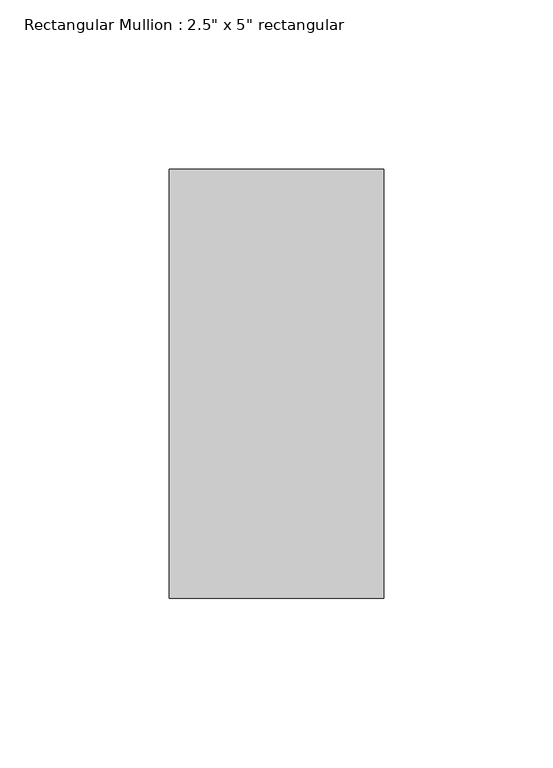
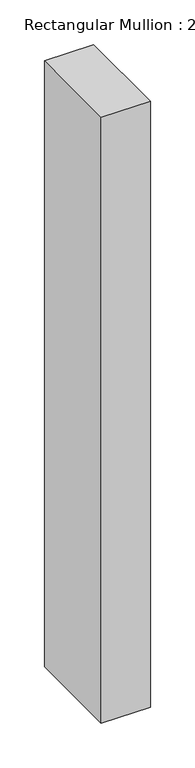
"""IFC4 building model written with IfcOpenShell, lengths in millimetres: member geometry."""

from ifc_helpers import new_model, si_unit, frame, origin, place, context, project, spatial, polyline, outline, extrude, source, transform, mapped, element, save


def member_3519937d(model_context):
    return source(origin(), model_context, "Body", "SweptSolid", [
        extrude(outline(polyline([(0.0, 63.5), (0.0, -63.5), (-63.5, -63.5), (-63.5, 63.5), (0.0, 63.5)])), frame((0.0, 0.0, -827.5712747), z_axis=(0.0, 0.0, 1.0), x_axis=(1.0, 0.0, 0.0)), (0.0, 0.0, 1.0), 827.5712747),
    ])


if __name__ == "__main__":
    model = new_model("IFC4")
    model_context = context("Model", 3, world=origin())
    ifc_project = project(units=[si_unit("LENGTHUNIT", "METRE", prefix="MILLI")], contexts=[model_context])
    site = spatial("IfcSite", under=ifc_project)
    building = spatial("IfcBuilding", under=site)
    placement = place(None, origin())
    member_shape = member_3519937d(model_context)
    element("IfcMember", 1, ObjectType="Rectangular Mullion : 2.5\" x 5\" rectangular", at=placement, inside=building, context=model_context, shape_type="MappedRepresentation", body=[
        mapped(member_shape, transform((0.0, 0.0, 0.0), x_axis=(1.0, 0.0, 0.0), y_axis=(0.0, 1.0, 0.0), z_axis=(0.0, 0.0, 1.0))),
    ])
    save(model, "model.ifc")

# Revit data of these elements
# Type "Rectangular Mullion : 2.5\" x 5\" rectangular"
#   built-in parameter 1007304 = 0.416667 (stored number, unit not read)
#   built-in parameter 1007301 = 0.104167 (stored number, unit not read)
#   built-in parameter 1007300 = 0.104167 (stored number, unit not read)
# Element 1 (IfcMember, "Rectangular Mullion : 2.5\" x 5\" rectangular")
#   Materials on its faces: "Aluminum"
# Materials
#   "Aluminum": class "Metal", colour RGB 247 247 247, transparency 0, Description = "Aluminum 6061", Cost = 0
